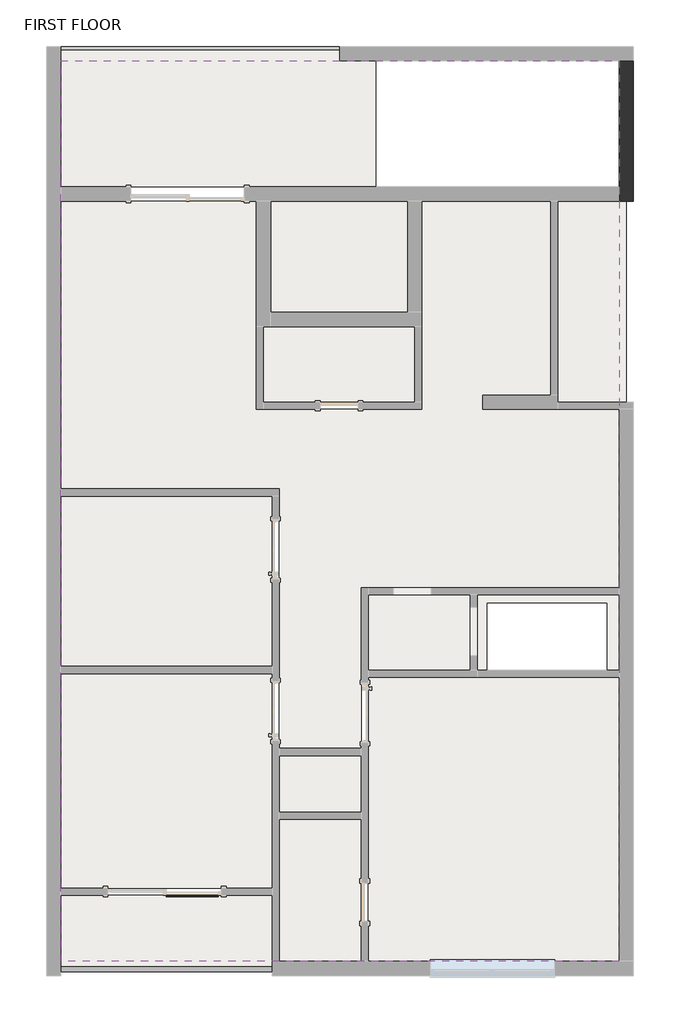
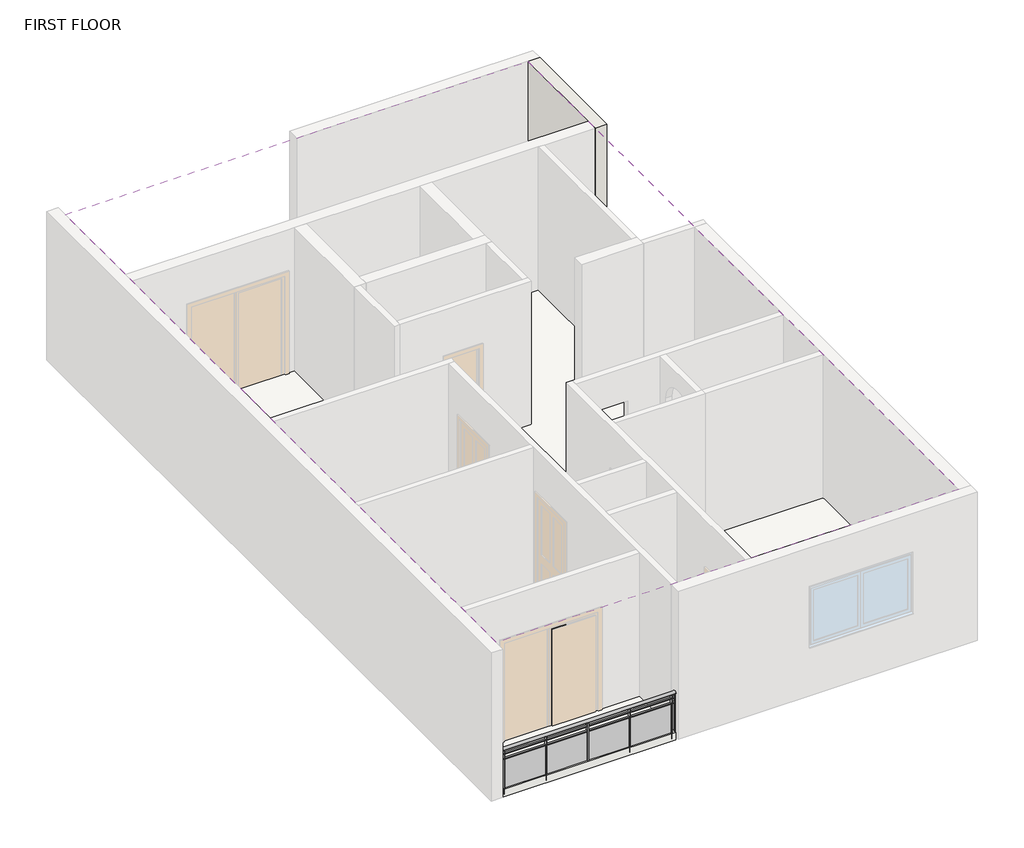
# One storey, part 2 of 2: 2 railings, 1 roof, 1 slab, 1 wall.
"""IFC4 building model written with IfcOpenShell, lengths in millimetres."""

from ifc_helpers import new_model, si_unit, point, frame, origin, place, context, project, spatial, polyline, ellipse_curve, trimmed, outline, extrude, faceted_brep, element, save
from ifc_brep_helpers import plane_surface, extruded_surface, advanced_brep

model = new_model("IFC4")

# Units and contexts
model_context = context("Model", 3, world=origin())
ifc_project = project(units=[si_unit("LENGTHUNIT", "METRE", prefix="MILLI")], contexts=[model_context])

# Site, building, storey
site = spatial("IfcSite", under=ifc_project)
building = spatial("IfcBuilding", under=site)
storey = spatial("IfcBuildingStorey", under=building, Name="FIRST FLOOR", Elevation=3352.8)

# Railings
placement = place(None, origin())
element("IfcRailing", 1, ObjectType="Glass Panel - Bottom Fill", at=placement, inside=storey, context=model_context, shape_type="SolidModel", body=[
    advanced_brep(
    [(-18145.1229553, -6923.8035687, 4267.2), (-18145.1229553, -7000.0035687, 4267.2), (-14741.5229553, -6923.8035687, 4267.2), (-14741.5229553, -7000.0035687, 4267.2)],
    [
        (0, 1, ellipse_curve(frame((-18145.1229553, -6961.9035687, 4267.2), z_axis=(-1.0, 0.0, 0.0), x_axis=(0.0, -1.0, 0.0)), 38.1, 28.575)),
        (1, 0, ellipse_curve(frame((-18145.1229553, -6961.9035687, 4267.2), z_axis=(-1.0, 0.0, 0.0), x_axis=(0.0, -1.0, 0.0)), 38.1, 28.575)),
        (2, 3, ellipse_curve(frame((-14741.5229553, -6961.9035687, 4267.2), z_axis=(1.0, 0.0, 0.0), x_axis=(0.0, -1.0, 0.0)), 38.1, 28.575)),
        (3, 2, ellipse_curve(frame((-14741.5229553, -6961.9035687, 4267.2), z_axis=(1.0, 0.0, 0.0), x_axis=(0.0, -1.0, 0.0)), 38.1, 28.575)),
        (0, 2),
        (3, 1),
    ],
    [
        plane_surface(frame((-18145.1229553, -6961.9035687, 4267.2), z_axis=(-1.0, 0.0, 0.0), x_axis=(0.0, 1.0, 0.0))),
        plane_surface(frame((-14741.5229553, -6961.9035687, 4267.2), z_axis=(1.0, 0.0, 0.0), x_axis=(0.0, 1.0, 0.0))),
        extruded_surface(trimmed(ellipse_curve(frame((-14741.5229553, -6961.9035687, 4267.2), z_axis=(-1.0, 0.0, 0.0), x_axis=(0.0, -1.0, 0.0)), 38.1, 28.575), [point((-14741.5229553, -6923.8035687, 4267.2))], [point((-14741.5229553, -7000.0035687, 4267.2))], True, "CARTESIAN"), (-3403.6000000000004, 0.0, 0.0), 3403.6000000000004),
        extruded_surface(trimmed(ellipse_curve(frame((-14741.5229553, -6961.9035687, 4267.2), z_axis=(-1.0, 0.0, 0.0), x_axis=(0.0, -1.0, 0.0)), 38.1, 28.575), [point((-14741.5229553, -7000.0035687, 4267.2))], [point((-14741.5229553, -6923.8035687, 4267.2))], True, "CARTESIAN"), (-3403.6000000000004, 0.0, 0.0), 3403.6000000000004),
    ],
    [
        (0, [[1, 2]]),
        (1, [[3, 4]]),
        (2, [[-1, 5, -4, 6]]),
        (3, [[-2, -6, -3, -5]]),
    ],
),
    extrude(outline(polyline([(-18145.1229553, -6974.6035687), (-18145.1229553, -6949.2035687), (-14741.5229553, -6949.2035687), (-14741.5229553, -6974.6035687), (-18145.1229553, -6974.6035687)])), frame((0.0, 0.0, 4152.9), z_axis=(0.0, 0.0, 1.0), x_axis=(1.0, 0.0, 0.0)), (0.0, 0.0, 1.0), 25.4),
    extrude(outline(polyline([(-18145.1229553, -6974.6035687), (-18145.1229553, -6949.2035687), (-14741.5229553, -6949.2035687), (-14741.5229553, -6974.6035687), (-18145.1229553, -6974.6035687)])), frame((0.0, 0.0, 4051.3), z_axis=(0.0, 0.0, 1.0), x_axis=(1.0, 0.0, 0.0)), (0.0, 0.0, 1.0), 25.4),
    extrude(outline(polyline([(-14824.0729553, -6987.3035687), (-14824.0729553, -6936.5035687), (-14811.3729553, -6936.5035687), (-14811.3729553, -6987.3035687), (-14824.0729553, -6987.3035687)])), frame((0.0, 0.0, 3352.8), z_axis=(0.0, 0.0, 1.0), x_axis=(1.0, 0.0, 0.0)), (0.0, 0.0, 1.0), 885.825),
    extrude(outline(polyline([(-15630.5229553, -6955.3684117), (-14817.7229553, -6955.3684117), (-14817.7229553, -6961.7184117), (-15630.5229553, -6961.7184117), (-15630.5229553, -6955.3684117)])), frame((0.0, 0.0, 3454.4), z_axis=(0.0, 0.0, 1.0), x_axis=(1.0, 0.0, 0.0)), (0.0, 0.0, 1.0), 596.9),
    extrude(outline(polyline([(-15636.8729553, -6987.3035687), (-15636.8729553, -6936.5035687), (-15624.1729553, -6936.5035687), (-15624.1729553, -6987.3035687), (-15636.8729553, -6987.3035687)])), frame((0.0, 0.0, 3352.8), z_axis=(0.0, 0.0, 1.0), x_axis=(1.0, 0.0, 0.0)), (0.0, 0.0, 1.0), 885.825),
    extrude(outline(polyline([(-16443.3229553, -6955.3684117), (-15630.5229553, -6955.3684117), (-15630.5229553, -6961.7184117), (-16443.3229553, -6961.7184117), (-16443.3229553, -6955.3684117)])), frame((0.0, 0.0, 3454.4), z_axis=(0.0, 0.0, 1.0), x_axis=(1.0, 0.0, 0.0)), (0.0, 0.0, 1.0), 596.9),
    extrude(outline(polyline([(-16449.6729553, -6987.3035687), (-16449.6729553, -6936.5035687), (-16436.9729553, -6936.5035687), (-16436.9729553, -6987.3035687), (-16449.6729553, -6987.3035687)])), frame((0.0, 0.0, 3352.8), z_axis=(0.0, 0.0, 1.0), x_axis=(1.0, 0.0, 0.0)), (0.0, 0.0, 1.0), 885.825),
    extrude(outline(polyline([(-17256.1229553, -6955.3684117), (-16443.3229553, -6955.3684117), (-16443.3229553, -6961.7184117), (-17256.1229553, -6961.7184117), (-17256.1229553, -6955.3684117)])), frame((0.0, 0.0, 3454.4), z_axis=(0.0, 0.0, 1.0), x_axis=(1.0, 0.0, 0.0)), (0.0, 0.0, 1.0), 596.9),
    extrude(outline(polyline([(-17262.4729553, -6987.3035687), (-17262.4729553, -6936.5035687), (-17249.7729553, -6936.5035687), (-17249.7729553, -6987.3035687), (-17262.4729553, -6987.3035687)])), frame((0.0, 0.0, 3352.8), z_axis=(0.0, 0.0, 1.0), x_axis=(1.0, 0.0, 0.0)), (0.0, 0.0, 1.0), 885.825),
    extrude(outline(polyline([(-18068.9229553, -6955.3684117), (-17256.1229553, -6955.3684117), (-17256.1229553, -6961.7184117), (-18068.9229553, -6961.7184117), (-18068.9229553, -6955.3684117)])), frame((0.0, 0.0, 3454.4), z_axis=(0.0, 0.0, 1.0), x_axis=(1.0, 0.0, 0.0)), (0.0, 0.0, 1.0), 596.9),
    extrude(outline(polyline([(-18075.2729553, -6987.3035687), (-18075.2729553, -6936.5035687), (-18062.5729553, -6936.5035687), (-18062.5729553, -6987.3035687), (-18075.2729553, -6987.3035687)])), frame((0.0, 0.0, 3352.8), z_axis=(0.0, 0.0, 1.0), x_axis=(1.0, 0.0, 0.0)), (0.0, 0.0, 1.0), 885.825),
    extrude(outline(polyline([(-14754.2229553, -6971.4285687), (-14754.2229553, -6952.3785687), (-14735.1729553, -6952.3785687), (-14735.1729553, -6971.4285687), (-14754.2229553, -6971.4285687)])), frame((0.0, 0.0, 3352.8), z_axis=(0.0, 0.0, 1.0), x_axis=(1.0, 0.0, 0.0)), (0.0, 0.0, 1.0), 885.825),
    extrude(outline(polyline([(-18151.4729553, -6971.4285687), (-18151.4729553, -6952.3785687), (-18132.4229553, -6952.3785687), (-18132.4229553, -6971.4285687), (-18151.4729553, -6971.4285687)])), frame((0.0, 0.0, 3352.8), z_axis=(0.0, 0.0, 1.0), x_axis=(1.0, 0.0, 0.0)), (0.0, 0.0, 1.0), 885.825),
])
element("IfcRailing", 2, ObjectType="Handrail - Rectangular", at=placement, inside=storey, context=model_context, shape_type="SweptSolid", body=[
    extrude(outline(polyline([(-18145.1229553, 7846.2964313), (-18145.1229553, 7897.0964313), (-13649.3229553, 7897.0964313), (-13649.3229553, 7846.2964313), (-18145.1229553, 7846.2964313)])), frame((0.0, 0.0, 4216.4), z_axis=(0.0, 0.0, 1.0), x_axis=(1.0, 0.0, 0.0)), (0.0, 0.0, 1.0), 50.8),
    extrude(outline(polyline([(-13684.2479553, 7862.1714313), (-13684.2479553, 7881.2214313), (-13665.1979553, 7881.2214313), (-13665.1979553, 7862.1714313), (-13684.2479553, 7862.1714313)])), frame((0.0, 0.0, 3352.8), z_axis=(0.0, 0.0, 1.0), x_axis=(1.0, 0.0, 0.0)), (0.0, 0.0, 1.0), 863.6),
    extrude(outline(polyline([(-13785.8479553, 7862.1714313), (-13785.8479553, 7881.2214313), (-13766.7979553, 7881.2214313), (-13766.7979553, 7862.1714313), (-13785.8479553, 7862.1714313)])), frame((0.0, 0.0, 3352.8), z_axis=(0.0, 0.0, 1.0), x_axis=(1.0, 0.0, 0.0)), (0.0, 0.0, 1.0), 863.6),
    extrude(outline(polyline([(-13887.4479553, 7862.1714313), (-13887.4479553, 7881.2214313), (-13868.3979553, 7881.2214313), (-13868.3979553, 7862.1714313), (-13887.4479553, 7862.1714313)])), frame((0.0, 0.0, 3352.8), z_axis=(0.0, 0.0, 1.0), x_axis=(1.0, 0.0, 0.0)), (0.0, 0.0, 1.0), 863.6),
    extrude(outline(polyline([(-13989.0479553, 7862.1714313), (-13989.0479553, 7881.2214313), (-13969.9979553, 7881.2214313), (-13969.9979553, 7862.1714313), (-13989.0479553, 7862.1714313)])), frame((0.0, 0.0, 3352.8), z_axis=(0.0, 0.0, 1.0), x_axis=(1.0, 0.0, 0.0)), (0.0, 0.0, 1.0), 863.6),
    extrude(outline(polyline([(-14090.6479553, 7862.1714313), (-14090.6479553, 7881.2214313), (-14071.5979553, 7881.2214313), (-14071.5979553, 7862.1714313), (-14090.6479553, 7862.1714313)])), frame((0.0, 0.0, 3352.8), z_axis=(0.0, 0.0, 1.0), x_axis=(1.0, 0.0, 0.0)), (0.0, 0.0, 1.0), 863.6),
    extrude(outline(polyline([(-14192.2479553, 7862.1714313), (-14192.2479553, 7881.2214313), (-14173.1979553, 7881.2214313), (-14173.1979553, 7862.1714313), (-14192.2479553, 7862.1714313)])), frame((0.0, 0.0, 3352.8), z_axis=(0.0, 0.0, 1.0), x_axis=(1.0, 0.0, 0.0)), (0.0, 0.0, 1.0), 863.6),
    extrude(outline(polyline([(-14293.8479553, 7862.1714313), (-14293.8479553, 7881.2214313), (-14274.7979553, 7881.2214313), (-14274.7979553, 7862.1714313), (-14293.8479553, 7862.1714313)])), frame((0.0, 0.0, 3352.8), z_axis=(0.0, 0.0, 1.0), x_axis=(1.0, 0.0, 0.0)), (0.0, 0.0, 1.0), 863.6),
    extrude(outline(polyline([(-14395.4479553, 7862.1714313), (-14395.4479553, 7881.2214313), (-14376.3979553, 7881.2214313), (-14376.3979553, 7862.1714313), (-14395.4479553, 7862.1714313)])), frame((0.0, 0.0, 3352.8), z_axis=(0.0, 0.0, 1.0), x_axis=(1.0, 0.0, 0.0)), (0.0, 0.0, 1.0), 863.6),
    extrude(outline(polyline([(-14497.0479553, 7862.1714313), (-14497.0479553, 7881.2214313), (-14477.9979553, 7881.2214313), (-14477.9979553, 7862.1714313), (-14497.0479553, 7862.1714313)])), frame((0.0, 0.0, 3352.8), z_axis=(0.0, 0.0, 1.0), x_axis=(1.0, 0.0, 0.0)), (0.0, 0.0, 1.0), 863.6),
    extrude(outline(polyline([(-14598.6479553, 7862.1714313), (-14598.6479553, 7881.2214313), (-14579.5979553, 7881.2214313), (-14579.5979553, 7862.1714313), (-14598.6479553, 7862.1714313)])), frame((0.0, 0.0, 3352.8), z_axis=(0.0, 0.0, 1.0), x_axis=(1.0, 0.0, 0.0)), (0.0, 0.0, 1.0), 863.6),
    extrude(outline(polyline([(-14700.2479553, 7862.1714313), (-14700.2479553, 7881.2214313), (-14681.1979553, 7881.2214313), (-14681.1979553, 7862.1714313), (-14700.2479553, 7862.1714313)])), frame((0.0, 0.0, 3352.8), z_axis=(0.0, 0.0, 1.0), x_axis=(1.0, 0.0, 0.0)), (0.0, 0.0, 1.0), 863.6),
    extrude(outline(polyline([(-14801.8479553, 7862.1714313), (-14801.8479553, 7881.2214313), (-14782.7979553, 7881.2214313), (-14782.7979553, 7862.1714313), (-14801.8479553, 7862.1714313)])), frame((0.0, 0.0, 3352.8), z_axis=(0.0, 0.0, 1.0), x_axis=(1.0, 0.0, 0.0)), (0.0, 0.0, 1.0), 863.6),
    extrude(outline(polyline([(-14903.4479553, 7862.1714313), (-14903.4479553, 7881.2214313), (-14884.3979553, 7881.2214313), (-14884.3979553, 7862.1714313), (-14903.4479553, 7862.1714313)])), frame((0.0, 0.0, 3352.8), z_axis=(0.0, 0.0, 1.0), x_axis=(1.0, 0.0, 0.0)), (0.0, 0.0, 1.0), 863.6),
    extrude(outline(polyline([(-15005.0479553, 7862.1714313), (-15005.0479553, 7881.2214313), (-14985.9979553, 7881.2214313), (-14985.9979553, 7862.1714313), (-15005.0479553, 7862.1714313)])), frame((0.0, 0.0, 3352.8), z_axis=(0.0, 0.0, 1.0), x_axis=(1.0, 0.0, 0.0)), (0.0, 0.0, 1.0), 863.6),
    extrude(outline(polyline([(-15106.6479553, 7862.1714313), (-15106.6479553, 7881.2214313), (-15087.5979553, 7881.2214313), (-15087.5979553, 7862.1714313), (-15106.6479553, 7862.1714313)])), frame((0.0, 0.0, 3352.8), z_axis=(0.0, 0.0, 1.0), x_axis=(1.0, 0.0, 0.0)), (0.0, 0.0, 1.0), 863.6),
    extrude(outline(polyline([(-15208.2479553, 7862.1714313), (-15208.2479553, 7881.2214313), (-15189.1979553, 7881.2214313), (-15189.1979553, 7862.1714313), (-15208.2479553, 7862.1714313)])), frame((0.0, 0.0, 3352.8), z_axis=(0.0, 0.0, 1.0), x_axis=(1.0, 0.0, 0.0)), (0.0, 0.0, 1.0), 863.6),
    extrude(outline(polyline([(-15309.8479553, 7862.1714313), (-15309.8479553, 7881.2214313), (-15290.7979553, 7881.2214313), (-15290.7979553, 7862.1714313), (-15309.8479553, 7862.1714313)])), frame((0.0, 0.0, 3352.8), z_axis=(0.0, 0.0, 1.0), x_axis=(1.0, 0.0, 0.0)), (0.0, 0.0, 1.0), 863.6),
    extrude(outline(polyline([(-15411.4479553, 7862.1714313), (-15411.4479553, 7881.2214313), (-15392.3979553, 7881.2214313), (-15392.3979553, 7862.1714313), (-15411.4479553, 7862.1714313)])), frame((0.0, 0.0, 3352.8), z_axis=(0.0, 0.0, 1.0), x_axis=(1.0, 0.0, 0.0)), (0.0, 0.0, 1.0), 863.6),
    extrude(outline(polyline([(-15513.0479553, 7862.1714313), (-15513.0479553, 7881.2214313), (-15493.9979553, 7881.2214313), (-15493.9979553, 7862.1714313), (-15513.0479553, 7862.1714313)])), frame((0.0, 0.0, 3352.8), z_axis=(0.0, 0.0, 1.0), x_axis=(1.0, 0.0, 0.0)), (0.0, 0.0, 1.0), 863.6),
    extrude(outline(polyline([(-15614.6479553, 7862.1714313), (-15614.6479553, 7881.2214313), (-15595.5979553, 7881.2214313), (-15595.5979553, 7862.1714313), (-15614.6479553, 7862.1714313)])), frame((0.0, 0.0, 3352.8), z_axis=(0.0, 0.0, 1.0), x_axis=(1.0, 0.0, 0.0)), (0.0, 0.0, 1.0), 863.6),
    extrude(outline(polyline([(-15716.2479553, 7862.1714313), (-15716.2479553, 7881.2214313), (-15697.1979553, 7881.2214313), (-15697.1979553, 7862.1714313), (-15716.2479553, 7862.1714313)])), frame((0.0, 0.0, 3352.8), z_axis=(0.0, 0.0, 1.0), x_axis=(1.0, 0.0, 0.0)), (0.0, 0.0, 1.0), 863.6),
    extrude(outline(polyline([(-15817.8479553, 7862.1714313), (-15817.8479553, 7881.2214313), (-15798.7979553, 7881.2214313), (-15798.7979553, 7862.1714313), (-15817.8479553, 7862.1714313)])), frame((0.0, 0.0, 3352.8), z_axis=(0.0, 0.0, 1.0), x_axis=(1.0, 0.0, 0.0)), (0.0, 0.0, 1.0), 863.6),
    extrude(outline(polyline([(-15919.4479553, 7862.1714313), (-15919.4479553, 7881.2214313), (-15900.3979553, 7881.2214313), (-15900.3979553, 7862.1714313), (-15919.4479553, 7862.1714313)])), frame((0.0, 0.0, 3352.8), z_axis=(0.0, 0.0, 1.0), x_axis=(1.0, 0.0, 0.0)), (0.0, 0.0, 1.0), 863.6),
    extrude(outline(polyline([(-16021.0479553, 7862.1714313), (-16021.0479553, 7881.2214313), (-16001.9979553, 7881.2214313), (-16001.9979553, 7862.1714313), (-16021.0479553, 7862.1714313)])), frame((0.0, 0.0, 3352.8), z_axis=(0.0, 0.0, 1.0), x_axis=(1.0, 0.0, 0.0)), (0.0, 0.0, 1.0), 863.6),
    extrude(outline(polyline([(-16122.6479553, 7862.1714313), (-16122.6479553, 7881.2214313), (-16103.5979553, 7881.2214313), (-16103.5979553, 7862.1714313), (-16122.6479553, 7862.1714313)])), frame((0.0, 0.0, 3352.8), z_axis=(0.0, 0.0, 1.0), x_axis=(1.0, 0.0, 0.0)), (0.0, 0.0, 1.0), 863.6),
    extrude(outline(polyline([(-16224.2479553, 7862.1714313), (-16224.2479553, 7881.2214313), (-16205.1979553, 7881.2214313), (-16205.1979553, 7862.1714313), (-16224.2479553, 7862.1714313)])), frame((0.0, 0.0, 3352.8), z_axis=(0.0, 0.0, 1.0), x_axis=(1.0, 0.0, 0.0)), (0.0, 0.0, 1.0), 863.6),
    extrude(outline(polyline([(-16325.8479553, 7862.1714313), (-16325.8479553, 7881.2214313), (-16306.7979553, 7881.2214313), (-16306.7979553, 7862.1714313), (-16325.8479553, 7862.1714313)])), frame((0.0, 0.0, 3352.8), z_axis=(0.0, 0.0, 1.0), x_axis=(1.0, 0.0, 0.0)), (0.0, 0.0, 1.0), 863.6),
    extrude(outline(polyline([(-16427.4479553, 7862.1714313), (-16427.4479553, 7881.2214313), (-16408.3979553, 7881.2214313), (-16408.3979553, 7862.1714313), (-16427.4479553, 7862.1714313)])), frame((0.0, 0.0, 3352.8), z_axis=(0.0, 0.0, 1.0), x_axis=(1.0, 0.0, 0.0)), (0.0, 0.0, 1.0), 863.6),
    extrude(outline(polyline([(-16529.0479553, 7862.1714313), (-16529.0479553, 7881.2214313), (-16509.9979553, 7881.2214313), (-16509.9979553, 7862.1714313), (-16529.0479553, 7862.1714313)])), frame((0.0, 0.0, 3352.8), z_axis=(0.0, 0.0, 1.0), x_axis=(1.0, 0.0, 0.0)), (0.0, 0.0, 1.0), 863.6),
    extrude(outline(polyline([(-16630.6479553, 7862.1714313), (-16630.6479553, 7881.2214313), (-16611.5979553, 7881.2214313), (-16611.5979553, 7862.1714313), (-16630.6479553, 7862.1714313)])), frame((0.0, 0.0, 3352.8), z_axis=(0.0, 0.0, 1.0), x_axis=(1.0, 0.0, 0.0)), (0.0, 0.0, 1.0), 863.6),
    extrude(outline(polyline([(-16732.2479553, 7862.1714313), (-16732.2479553, 7881.2214313), (-16713.1979553, 7881.2214313), (-16713.1979553, 7862.1714313), (-16732.2479553, 7862.1714313)])), frame((0.0, 0.0, 3352.8), z_axis=(0.0, 0.0, 1.0), x_axis=(1.0, 0.0, 0.0)), (0.0, 0.0, 1.0), 863.6),
    extrude(outline(polyline([(-16833.8479553, 7862.1714313), (-16833.8479553, 7881.2214313), (-16814.7979553, 7881.2214313), (-16814.7979553, 7862.1714313), (-16833.8479553, 7862.1714313)])), frame((0.0, 0.0, 3352.8), z_axis=(0.0, 0.0, 1.0), x_axis=(1.0, 0.0, 0.0)), (0.0, 0.0, 1.0), 863.6),
    extrude(outline(polyline([(-16935.4479553, 7862.1714313), (-16935.4479553, 7881.2214313), (-16916.3979553, 7881.2214313), (-16916.3979553, 7862.1714313), (-16935.4479553, 7862.1714313)])), frame((0.0, 0.0, 3352.8), z_axis=(0.0, 0.0, 1.0), x_axis=(1.0, 0.0, 0.0)), (0.0, 0.0, 1.0), 863.6),
    extrude(outline(polyline([(-17037.0479553, 7862.1714313), (-17037.0479553, 7881.2214313), (-17017.9979553, 7881.2214313), (-17017.9979553, 7862.1714313), (-17037.0479553, 7862.1714313)])), frame((0.0, 0.0, 3352.8), z_axis=(0.0, 0.0, 1.0), x_axis=(1.0, 0.0, 0.0)), (0.0, 0.0, 1.0), 863.6),
    extrude(outline(polyline([(-17138.6479553, 7862.1714313), (-17138.6479553, 7881.2214313), (-17119.5979553, 7881.2214313), (-17119.5979553, 7862.1714313), (-17138.6479553, 7862.1714313)])), frame((0.0, 0.0, 3352.8), z_axis=(0.0, 0.0, 1.0), x_axis=(1.0, 0.0, 0.0)), (0.0, 0.0, 1.0), 863.6),
    extrude(outline(polyline([(-17240.2479553, 7862.1714313), (-17240.2479553, 7881.2214313), (-17221.1979553, 7881.2214313), (-17221.1979553, 7862.1714313), (-17240.2479553, 7862.1714313)])), frame((0.0, 0.0, 3352.8), z_axis=(0.0, 0.0, 1.0), x_axis=(1.0, 0.0, 0.0)), (0.0, 0.0, 1.0), 863.6),
    extrude(outline(polyline([(-17341.8479553, 7862.1714313), (-17341.8479553, 7881.2214313), (-17322.7979553, 7881.2214313), (-17322.7979553, 7862.1714313), (-17341.8479553, 7862.1714313)])), frame((0.0, 0.0, 3352.8), z_axis=(0.0, 0.0, 1.0), x_axis=(1.0, 0.0, 0.0)), (0.0, 0.0, 1.0), 863.6),
    extrude(outline(polyline([(-17443.4479553, 7862.1714313), (-17443.4479553, 7881.2214313), (-17424.3979553, 7881.2214313), (-17424.3979553, 7862.1714313), (-17443.4479553, 7862.1714313)])), frame((0.0, 0.0, 3352.8), z_axis=(0.0, 0.0, 1.0), x_axis=(1.0, 0.0, 0.0)), (0.0, 0.0, 1.0), 863.6),
    extrude(outline(polyline([(-17545.0479553, 7862.1714313), (-17545.0479553, 7881.2214313), (-17525.9979553, 7881.2214313), (-17525.9979553, 7862.1714313), (-17545.0479553, 7862.1714313)])), frame((0.0, 0.0, 3352.8), z_axis=(0.0, 0.0, 1.0), x_axis=(1.0, 0.0, 0.0)), (0.0, 0.0, 1.0), 863.6),
    extrude(outline(polyline([(-17646.6479553, 7862.1714313), (-17646.6479553, 7881.2214313), (-17627.5979553, 7881.2214313), (-17627.5979553, 7862.1714313), (-17646.6479553, 7862.1714313)])), frame((0.0, 0.0, 3352.8), z_axis=(0.0, 0.0, 1.0), x_axis=(1.0, 0.0, 0.0)), (0.0, 0.0, 1.0), 863.6),
    extrude(outline(polyline([(-17748.2479553, 7862.1714313), (-17748.2479553, 7881.2214313), (-17729.1979553, 7881.2214313), (-17729.1979553, 7862.1714313), (-17748.2479553, 7862.1714313)])), frame((0.0, 0.0, 3352.8), z_axis=(0.0, 0.0, 1.0), x_axis=(1.0, 0.0, 0.0)), (0.0, 0.0, 1.0), 863.6),
    extrude(outline(polyline([(-17849.8479553, 7862.1714313), (-17849.8479553, 7881.2214313), (-17830.7979553, 7881.2214313), (-17830.7979553, 7862.1714313), (-17849.8479553, 7862.1714313)])), frame((0.0, 0.0, 3352.8), z_axis=(0.0, 0.0, 1.0), x_axis=(1.0, 0.0, 0.0)), (0.0, 0.0, 1.0), 863.6),
    extrude(outline(polyline([(-17951.4479553, 7862.1714313), (-17951.4479553, 7881.2214313), (-17932.3979553, 7881.2214313), (-17932.3979553, 7862.1714313), (-17951.4479553, 7862.1714313)])), frame((0.0, 0.0, 3352.8), z_axis=(0.0, 0.0, 1.0), x_axis=(1.0, 0.0, 0.0)), (0.0, 0.0, 1.0), 863.6),
    extrude(outline(polyline([(-18053.0479553, 7862.1714313), (-18053.0479553, 7881.2214313), (-18033.9979553, 7881.2214313), (-18033.9979553, 7862.1714313), (-18053.0479553, 7862.1714313)])), frame((0.0, 0.0, 3352.8), z_axis=(0.0, 0.0, 1.0), x_axis=(1.0, 0.0, 0.0)), (0.0, 0.0, 1.0), 863.6),
    extrude(outline(polyline([(-13668.3729553, 7862.1714313), (-13668.3729553, 7881.2214313), (-13649.3229553, 7881.2214313), (-13649.3229553, 7862.1714313), (-13668.3729553, 7862.1714313)])), frame((0.0, 0.0, 3352.8), z_axis=(0.0, 0.0, 1.0), x_axis=(1.0, 0.0, 0.0)), (0.0, 0.0, 1.0), 863.6),
    extrude(outline(polyline([(-18145.1229553, 7862.1714313), (-18145.1229553, 7881.2214313), (-18126.0729553, 7881.2214313), (-18126.0729553, 7862.1714313), (-18145.1229553, 7862.1714313)])), frame((0.0, 0.0, 3352.8), z_axis=(0.0, 0.0, 1.0), x_axis=(1.0, 0.0, 0.0)), (0.0, 0.0, 1.0), 863.6),
])

# Roof
element("IfcRoof", 3, ObjectType="roofing", at=placement, inside=storey, context=model_context, shape_type="SweptSolid", body=[
    extrude(outline(polyline([(-9153.5229553, -6834.9035687), (-14627.2229553, -6834.9035687), (-18145.1229553, -6834.9035687), (-18145.1229553, 7668.4964313), (-9153.5229553, 7668.4964313), (-9153.5229553, -6834.9035687)])), frame((0.0, 0.0, 6400.8), z_axis=(0.0, 0.0, 1.0), x_axis=(1.0, 0.0, 0.0)), (0.0, 0.0, 1.0), 304.8),
])

# Slab
element("IfcSlab", 4, at=placement, inside=storey, context=model_context, shape_type="SweptSolid", body=[
    extrude(outline(polyline([(-12557.1229553, 5407.8964313), (-12557.1229553, 3617.1964313), (-14766.9229553, 3617.1964313), (-14766.9229553, 5407.8964313), (-12557.1229553, 5407.8964313)])), frame((0.0, 0.0, 3302.0), z_axis=(0.0, 0.0, 1.0), x_axis=(1.0, 0.0, 0.0)), (0.0, 0.0, 1.0), 152.4),
    extrude(outline(polyline([(-12442.8229553, 3388.5964313), (-12442.8229553, 2169.3964313), (-14881.2229553, 2169.3964313), (-14881.2229553, 3388.5964313), (-12442.8229553, 3388.5964313)])), frame((0.0, 0.0, 3302.0), z_axis=(0.0, 0.0, 1.0), x_axis=(1.0, 0.0, 0.0)), (0.0, 0.0, 1.0), 152.4),
    extrude(outline(polyline([(-9153.5229553, -6834.9035687), (-13192.1229553, -6834.9035687), (-13192.1229553, -2262.9035687), (-9153.5229553, -2262.9035687), (-9153.5229553, -6834.9035687)])), frame((0.0, 0.0, 3302.0), z_axis=(0.0, 0.0, 1.0), x_axis=(1.0, 0.0, 0.0)), (0.0, 0.0, 1.0), 152.4),
    extrude(outline(polyline([(-11553.8229553, -929.4035687), (-11553.8229553, -2148.6035687), (-13192.1229553, -2148.6035687), (-13192.1229553, -929.4035687), (-11553.8229553, -929.4035687)])), frame((0.0, 0.0, 3302.0), z_axis=(0.0, 0.0, 1.0), x_axis=(1.0, 0.0, 0.0)), (0.0, 0.0, 1.0), 152.4),
    extrude(outline(polyline([(-11439.5229553, -929.4035687), (-9153.5229553, -929.4035687), (-9153.5229553, -2148.6035687), (-9344.0229553, -2148.6035687), (-9344.0229553, -1056.4035687), (-11287.1229553, -1056.4035687), (-11287.1229553, -2148.6035687), (-11439.5229553, -2148.6035687), (-11439.5229553, -929.4035687)])), frame((0.0, 0.0, 3302.0), z_axis=(0.0, 0.0, 1.0), x_axis=(1.0, 0.0, 0.0)), (0.0, 0.0, 1.0), 152.4),
    extrude(outline(polyline([(-14741.5229553, 658.0964313), (-14741.5229553, -2085.1035687), (-18145.1229553, -2085.1035687), (-18145.1229553, 658.0964313), (-14741.5229553, 658.0964313)])), frame((0.0, 0.0, 3302.0), z_axis=(0.0, 0.0, 1.0), x_axis=(1.0, 0.0, 0.0)), (0.0, 0.0, 1.0), 152.4),
    extrude(outline(polyline([(-14741.5229553, -2199.4035687), (-14741.5229553, -5653.8035687), (-18145.1229553, -5653.8035687), (-18145.1229553, -2199.4035687), (-14741.5229553, -2199.4035687)])), frame((0.0, 0.0, 3302.0), z_axis=(0.0, 0.0, 1.0), x_axis=(1.0, 0.0, 0.0)), (0.0, 0.0, 1.0), 152.4),
    extrude(outline(polyline([(-14741.5229553, -5768.1035687), (-14741.5229553, -6987.3035687), (-18145.1229553, -6987.3035687), (-18145.1229553, -5768.1035687), (-14741.5229553, -5768.1035687)])), frame((0.0, 0.0, 3302.0), z_axis=(0.0, 0.0, 1.0), x_axis=(1.0, 0.0, 0.0)), (0.0, 0.0, 1.0), 152.4),
    extrude(outline(polyline([(-14627.2229553, -3520.2035687), (-13306.4229553, -3520.2035687), (-13306.4229553, -4434.6035687), (-14627.2229553, -4434.6035687), (-14627.2229553, -3520.2035687)])), frame((0.0, 0.0, 3302.0), z_axis=(0.0, 0.0, 1.0), x_axis=(1.0, 0.0, 0.0)), (0.0, 0.0, 1.0), 152.4),
    extrude(outline(polyline([(-13306.4229553, -4548.9035687), (-13306.4229553, -6834.9035687), (-14627.2229553, -6834.9035687), (-14627.2229553, -4548.9035687), (-13306.4229553, -4548.9035687)])), frame((0.0, 0.0, 3302.0), z_axis=(0.0, 0.0, 1.0), x_axis=(1.0, 0.0, 0.0)), (0.0, 0.0, 1.0), 152.4),
    extrude(outline(polyline([(-9039.2229553, 5407.8964313), (-9039.2229553, 2169.3964313), (-10144.1229553, 2169.3964313), (-10144.1229553, 5407.8964313), (-9039.2229553, 5407.8964313)])), frame((0.0, 0.0, 3302.0), z_axis=(0.0, 0.0, 1.0), x_axis=(1.0, 0.0, 0.0)), (0.0, 0.0, 1.0), 152.4),
    extrude(outline(polyline([(-13306.4229553, -3405.9035687), (-14627.2229553, -3405.9035687), (-14627.2229553, 772.3964313), (-18145.1229553, 772.3964313), (-18145.1229553, 5407.8964313), (-14995.5229553, 5407.8964313), (-14995.5229553, 2055.0964313), (-12328.5229553, 2055.0964313), (-12328.5229553, 5407.8964313), (-10258.4229553, 5407.8964313), (-10258.4229553, 2283.6964313), (-11350.6229553, 2283.6964313), (-11350.6229553, 2055.0964313), (-9153.5229553, 2055.0964313), (-9153.5229553, -815.1035687), (-13306.4229553, -815.1035687), (-13306.4229553, -3405.9035687)])), frame((0.0, 0.0, 3302.0), z_axis=(0.0, 0.0, 1.0), x_axis=(1.0, 0.0, 0.0)), (0.0, 0.0, 1.0), 152.4),
    extrude(outline(polyline([(-18145.1229553, 7846.2964313), (-13649.3229553, 7846.2964313), (-13649.3229553, 7668.4964313), (-13068.4571222, 7668.4964313), (-13068.4571222, 5636.4964313), (-18145.1229553, 5636.4964313), (-18145.1229553, 7846.2964313)])), frame((0.0, 0.0, 3302.0), z_axis=(0.0, 0.0, 1.0), x_axis=(1.0, 0.0, 0.0)), (0.0, 0.0, 1.0), 152.4),
])

# Wall
element("IfcWall", 5, ObjectType="EXTERIOR WALL 9\"", at=placement, inside=storey, context=model_context, shape_type="Brep", body=[
    faceted_brep([(-9153.5229553, 7668.4964313, 3352.8), (-9153.5229553, 5636.4964313, 3352.8), (-9153.5229553, 5407.8964313, 3352.8), (-9153.5229553, 5407.8964313, 6400.8), (-9153.5229553, 5636.4964313, 6400.8), (-9153.5229553, 7668.4964313, 6400.8), (-8924.9229553, 7668.4964313, 3352.8), (-8924.9229553, 7668.4964313, 6400.8), (-8924.9229553, 5407.8964313, 6400.8), (-8924.9229553, 5407.8964313, 3352.8)], [[[0, 1, 2, 3, 4, 5]], [[6, 7, 8, 9]], [[2, 1, 0, 6, 9]], [[5, 4, 3, 8, 7]], [[0, 5, 7, 6]], [[3, 2, 9, 8]]]),
])

save(model, "model.ifc")

# Revit data of these elements
# Type "Glass Panel - Bottom Fill"
#   Assembly Code = "C2010400"
#   built-in parameter 1008612 = 0.0416667 (stored number, unit not read)
#   built-in parameter 1008611 = 0.0416667 (stored number, unit not read)
#   built-in parameter 1008609 = 0.333333 (stored number, unit not read)
#   built-in parameter 1008604 = 0.166667 (stored number, unit not read)
#   built-in parameter 1008603 = 0.166667 (stored number, unit not read)
#   Railing Height = 3' - 0"
#   built-in parameter 1008630 = 2
#   built-in parameter 1008610 = 2
#   built-in parameter 1008618 = Baluster - Square : 3/4"
# Type "Handrail - Rectangular"
#   Assembly Code = "C2010400"
#   built-in parameter 1008612 = 0.0416667 (stored number, unit not read)
#   built-in parameter 1008611 = 0.0416667 (stored number, unit not read)
#   built-in parameter 1008609 = 0.333333 (stored number, unit not read)
#   built-in parameter 1008604 = 0.166667 (stored number, unit not read)
#   built-in parameter 1008603 = 0.166667 (stored number, unit not read)
#   Railing Height = 3' - 0"
#   built-in parameter 1008630 = 2
#   built-in parameter 1008610 = 2
#   built-in parameter 1008618 = Baluster - Square : 3/4"
# Type "roofing"
#   Assembly Code = "B1020"
#   Layers, outside or top first: 1' - 0" "ROOFING 1'" (function 1)
# Type
#   Assembly Code = "B1010"
#   Function = 0
#   Layers, outside or top first: 0' - 6" "MARBLE" (function 1)
# Type "EXTERIOR WALL 9\""
#   Assembly Code = "B2010"
#   Layers, outside or top first: 0' - 9" "EXTERIOR WALL WHITE COLOUR" (function 1)
# Element 1 (IfcRailing, "Glass Panel - Bottom Fill")
#   Phase Created = New Construction
#   Materials on its faces: "Glass"
# Element 2 (IfcRailing, "Handrail - Rectangular")
#   Phase Created = New Construction
# Element 3 (IfcRoof, "roofing")
#   built-in parameter 1001705 = 22 (stored number, unit not read)
#   built-in parameter 1001701 = 10 (stored number, unit not read)
#   built-in parameter 1001710 = 33615
#   Phase Created = New Construction
#   Materials on its faces: "ROOFING 1'"
# Element 4 (IfcSlab)
#   Height Offset From Level = 0' - 4"
#   Phase Created = New Construction
#   Materials on its faces: "MARBLE"
# Element 5 (IfcWall, "EXTERIOR WALL 9\"")
#   Top Offset = 0' - 0"
#   Base Offset = 0' - 0"
#   wall height = 10' - 0"
#   Phase Created = New Construction
#   Base Constraint = FIRST FLOOR
#   Top Constraint = SECOND FLR
#   Materials on its faces: "EXTERIOR WALL WHITE COLOUR"
# Materials
#   "ROOFING 1'": class "Generic", colour RGB 120 120 120, transparency 0, Cost = 0
#   "MARBLE": class "Generic", colour RGB 120 120 120, transparency 0, Cost = 0
#   "EXTERIOR WALL WHITE COLOUR": class "Generic", colour RGB 120 120 120, transparency 0, Cost = 0
#   "Glass": class "Glass", colour RGB 0 128 192, transparency 0.75, Description = "Soda Lime Glass", Cost = 0
